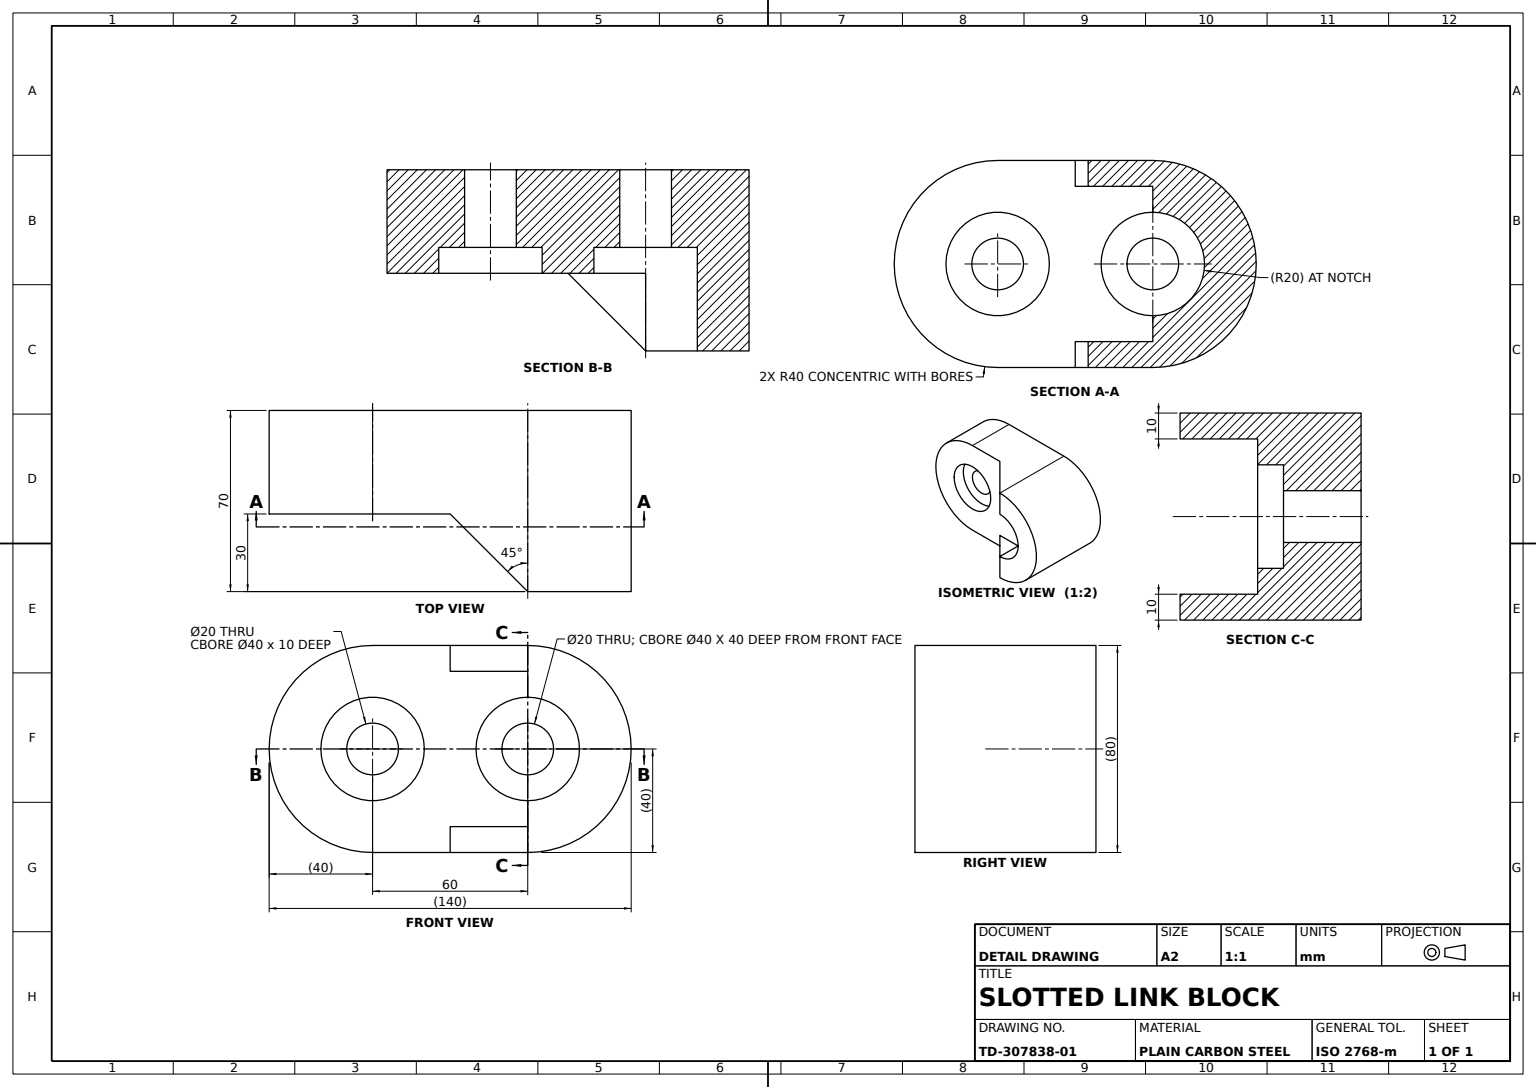
from build123d import *

# Parameters (mm, degrees)
BASE_BLOCK_80X80X40_DEPTH = 40
COUNTERBORE_1_SKETCH_R    = 20
COUNTERBORE_1_40X10_DEPTH = 10
BORE_1_SKETCH_R           = 10
BORE_1_20_DEPTH           = 30
SIDE_BOSS_DEPTH           = 30
SIDE_BOSS_TRIM_CUT_DEPTH  = 30
COUNTERBORE_2_SKETCH_R    = 20
COUNTERBORE_2_40X10_DEPTH = 10
BORE_2_SKETCH_R           = 10
BORE_2_20_DEPTH           = 30
GUSSET_1_DEPTH            = 10
GUSSET_2_DEPTH            = 10


with BuildPart() as part:
    # Base Block Sketch → Base Block 80x80x40 (new body)
    with BuildSketch(Plane.XY):
        with BuildLine():
            Line((0, 40), (60, 40))
            ThreePointArc((60, 40), (100, 0), (60, -40))
            Line((60, -40), (0, -40))
            ThreePointArc((0, -40), (-40, 0), (0, 40))
        make_face()
    extrude(amount=BASE_BLOCK_80X80X40_DEPTH)

    # Counterbore 1 Sketch → Counterbore 1 Ø40x10 (cut)
    with BuildSketch(Plane.XY.offset(40)):
        Circle(COUNTERBORE_1_SKETCH_R)
    extrude(amount=-COUNTERBORE_1_40X10_DEPTH, mode=Mode.SUBTRACT)

    # Bore 1 Sketch → Bore 1 Ø20 (cut)
    with BuildSketch(Plane.XY.offset(30)):
        Circle(BORE_1_SKETCH_R)
    extrude(amount=-BORE_1_20_DEPTH, mode=Mode.SUBTRACT)

    # Side Boss Sketch → Side Boss (add)
    with BuildSketch(Plane.XY.offset(40)):
        with BuildLine():
            Line((60, 40), (60, -40))
            ThreePointArc((60, -40), (100, 0), (60, 40))
        make_face()
    extrude(amount=SIDE_BOSS_DEPTH)

    # Side Boss Trim Sketch → Side Boss Trim Cut (cut)
    with BuildSketch(Plane.XY.offset(70)):
        with BuildLine():
            Line((60, 20), (60, -20))
            ThreePointArc((60, -20), (80, 0), (60, 20))
        make_face()
    extrude(amount=-SIDE_BOSS_TRIM_CUT_DEPTH, mode=Mode.SUBTRACT)

    # Counterbore 2 Sketch → Counterbore 2 Ø40x10 (cut)
    with BuildSketch(Plane.XY.offset(40)):
        with Locations((60, 0)):
            Circle(COUNTERBORE_2_SKETCH_R)
    extrude(amount=-COUNTERBORE_2_40X10_DEPTH, mode=Mode.SUBTRACT)

    # Bore 2 Sketch → Bore 2 Ø20 (cut)
    with BuildSketch(Plane.XY.offset(30)):
        with Locations((60, 0)):
            Circle(BORE_2_SKETCH_R)
    extrude(amount=-BORE_2_20_DEPTH, mode=Mode.SUBTRACT)

    # Gusset 1 Sketch → Gusset 1 (add)
    with BuildSketch(Plane.XZ.offset(40)):
        Polygon((60, 70), (60, 40), (30, 40), align=None)
    extrude(amount=-GUSSET_1_DEPTH)

    # Gusset 2 Sketch → Gusset 2 (add)
    with BuildSketch(Plane(origin=(0, 40, 0), x_dir=(1, 0, 0), z_dir=(0, 1, 0))):
        Polygon((60, -70), (60, -40), (30, -40), align=None)
    extrude(amount=-GUSSET_2_DEPTH)


solid = part.part
